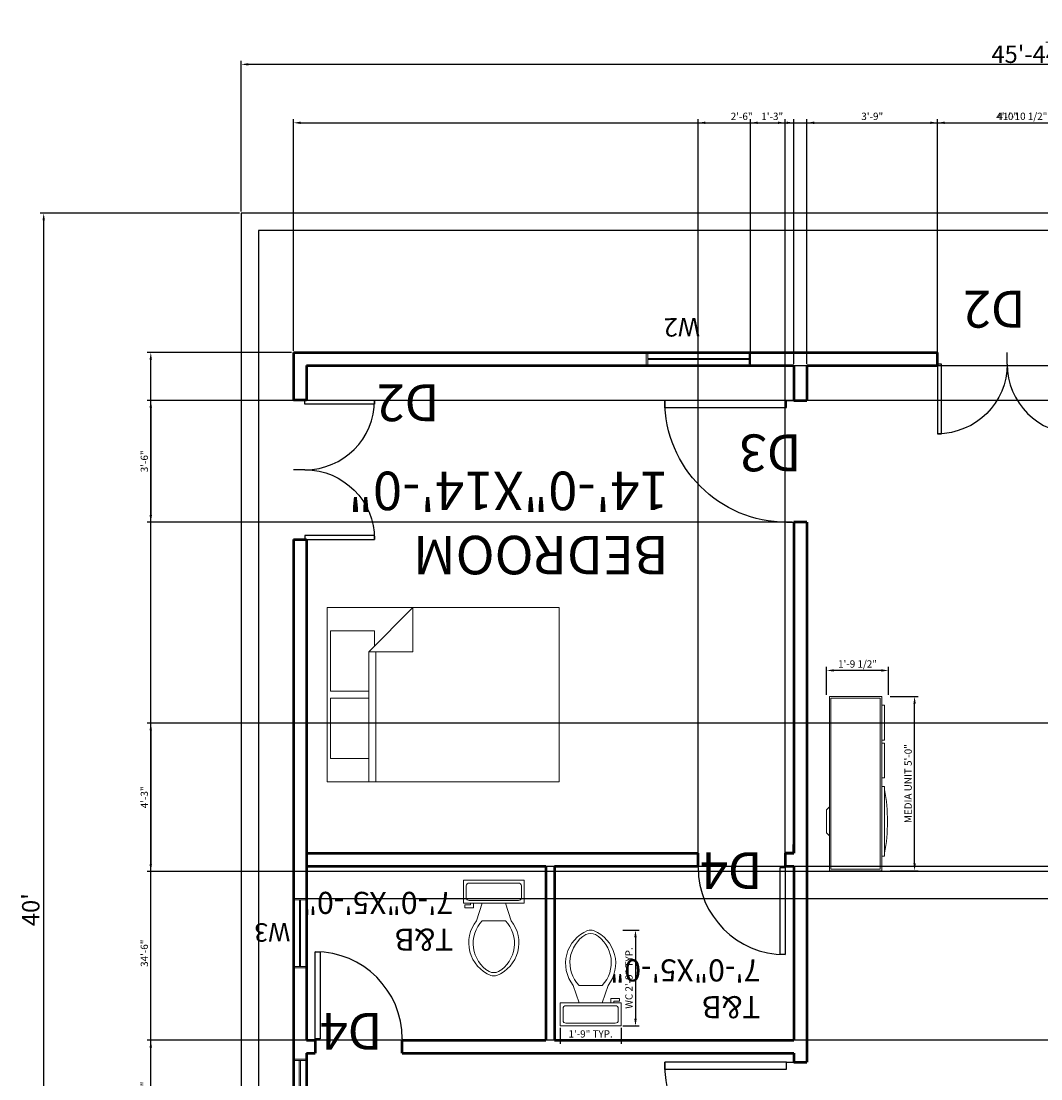
# Model space of a CAD drawing. Units: inches. Extents: x 1989 to 2637, y 1032 to 1611.
# Tile 2 of 5: x 1989 to 2340, y 1247 to 1611. Entities that reach past the tile are written whole.
import ezdxf

# ---------------------------------------------------------------- set-up
doc = ezdxf.new("R2010")
doc.units = ezdxf.units.IN
for name, color, linetype, lineweight in [('A-ANNO-TEXT', 1, 'Continuous', 18), ('A-AREA-IDEN', 1, 'Continuous', 25), ('A-FLOR-FIXT', 8, 'Continuous', 18), ('C-PROP', 7, 'Continuous', 25), ('DIMENSIONS', 7, 'Continuous', 18), ('doors', 5, 'Continuous', 25), ('furniture', 8, 'Continuous', 18), ('walls', 7, 'Continuous', 50), ('windows', 3, 'Continuous', 18)]:
    doc.layers.add(name, color=color, linetype=linetype, lineweight=lineweight)
doc.styles.get("Standard").update_dxf_attribs({"font": 'arial.ttf'})
doc.dimstyles.new('ISO-25', dxfattribs={"dimtxt": 2.5, "dimasz": 2.5, "dimexe": 1.25, "dimexo": 0.625, "dimtad": 1, "dimlunit": 4, "dimtxsty": 'Standard', "dimcen": 2.5, "dimadec": 0, "dimazin": 0, "dimtfac": 1, "dimtmove": 0, "dimatfit": 3, "dimfxl": 1, "dimarcsym": 0})

# ---------------------------------------------------------------- blocks, each defined once
blk = doc.blocks.new('*U2')
for p, q in [((0, 0), (0, -5)), ((30, 0), (30, -5))]:
    blk.add_line(p, q)
blk.add_lwpolyline([(0, 0), (0, 30), (1.75, 30), (1.75, 0)], close=True)
blk.add_arc((0, 0), 30, 0, 90)
blk = doc.blocks.new('Entertainment Center')
for p, q in [((-4, 0), (-5, -1)), ((4, 0), (-4, 0)), ((5, -1), (4, 0)), ((-17, -19), (-17, -1)), ((-17, -1), (43, -1)), ((-16.5, -18.5), (-16.5, -1.5)), ((-16.5, -1.5), (42.5, -1.5)), ((42.5, -1.5), (42.5, -18.5)), ((43, -1), (43, -19)), ((43, -19), (-17, -19)), ((42.5, -18.5), (-16.5, -18.5)), ((-12, -20), (-12, -19)), ((12, -20), (-12, -20)), ((12, -19), (12, -20)), ((15, -20), (15, -19)), ((27, -20), (15, -20)), ((27, -19), (27, -20)), ((28, -20), (28, -19)), ((40, -20), (28, -20)), ((40, -19), (40, -20))]:
    blk.add_line(p, q)
blk.add_arc((0, 40), 61, 259.6111, 280.3889)
blk = doc.blocks.new('Bed - Queen')
for p, q in [((0, -80.00003), (0, 0)), ((0, 0), (59.99999, 0)), ((59.99999, 0), (59.99999, -80.00003)), ((7.99999, -1.2), (28.79998, -1.2)), ((7.99999, -14.4), (7.99999, -1.2)), ((28.79998, -1.2), (28.79998, -14.4)), ((31.19999, -1.2), (51.99999, -1.2)), ((31.19999, -14.4), (31.19999, -1.2)), ((51.99999, -1.2), (51.99999, -16.4)), ((0, -14.4), (44.8, -14.4)), ((59.99999, -29.6), (44.8, -14.4)), ((44.8, -14.4), (44.8, -29.6)), ((44.8, -16.8), (0, -16.8)), ((51.99999, -16.4), (46.79936, -16.4)), ((44.8, -29.6), (59.99999, -29.6)), ((59.99999, -80.00003), (0, -80.00003))]:
    blk.add_line(p, q)
blk = doc.blocks.new('Toilet - top')
for p, q in [((9.5, -6), (9.5, -2)), ((-10, -8.5), (-8, -8.5)), ((-10, -9.5), (-10, -8.5)), ((-7, -9.5), (-10, -9.5)), ((-8, -8.5), (-8, -8)), ((-7, -8), (-7, -9.5)), ((-4, -8), (-6, -14)), ((4, -8), (6, -14)), ((4, -14), (-4, -14))]:
    blk.add_line(p, q)
blk.add_lwpolyline([(10.5, -8), (10.5, 0), (-10.5, 0), (-10.5, -8)], close=True)
for points in [[(-9.5, -2), (-9.5, -6)], [(8.5, -1), (-8.5, -1)], [(-8.5, -7), (8.5, -7)]]:
    blk.add_lwpolyline(points)
for centre, radius, start, end in [((-8.62, -1.88), 0.884, 81.8699, 188.1301), ((8.62, -1.88), 0.884, 351.8699, 98.1301), ((-8.62, -6.12), 0.884, 171.8699, 278.1301), ((8.62, -6.12), 0.884, 261.8699, 8.1301), ((3.52, -21.58), 12.17, 141.4691, 247.9714), ((4.2, -21.82), 11.33, 136.3677, 238.9468), ((-3.52, -21.58), 12.17, 292.0284, 38.5307), ((-4.2, -21.82), 11.33, 301.053, 43.6321), ((0, -27.88), 4, 245.7318, 294.2682), ((0, -29), 4, 254.8605, 285.1395)]:
    blk.add_arc(centre, radius, start, end)
blk = doc.blocks.new('*D11')
at = {"layer": 'Defpoints', "color": 0, "transparency": 16777216}
for p in [(1996.45, 1544.92), (2064.5, 1544.92), (2064.5, 1064.92)]:
    blk.add_point(p, dxfattribs=at)
at = {"layer": 'DIMENSIONS', "color": 0, "lineweight": -2, "transparency": 16777216}
for p, q in [((2063.87, 1544.92), (1995.2, 1544.92)), ((1996.45, 1067.42), (1996.45, 1542.42)), ((2063.87, 1064.92), (1995.2, 1064.92))]:
    blk.add_line(p, q, dxfattribs=at)
at = {"layer": 'DIMENSIONS', "color": 0, "transparency": 16777216}
for points in [[(1996.03, 1542.42), (1996.87, 1542.42), (1996.45, 1544.92)], [(1996.03, 1067.42), (1996.87, 1067.42), (1996.45, 1064.92)]]:
    blk.add_solid(points, dxfattribs=at)
at = {"layer": 'DIMENSIONS', "color": 0, "transparency": 16777216, "insert": (1992.76, 1304.92), "char_height": 6, "attachment_point": 5, "rotation": 90}
blk.add_mtext("40'", dxfattribs=at)
blk = doc.blocks.new('*D12')
at = {"layer": 'Defpoints', "color": 0, "transparency": 16777216}
for p in [(2064.5, 1596.21), (2064.5, 1544.92), (2608.81, 1544.92)]:
    blk.add_point(p, dxfattribs=at)
at = {"layer": 'DIMENSIONS', "color": 0, "lineweight": -2, "transparency": 16777216}
for p, q in [((2064.5, 1545.55), (2064.5, 1597.46)), ((2608.81, 1545.55), (2608.81, 1597.46)), ((2606.31, 1596.21), (2067, 1596.21))]:
    blk.add_line(p, q, dxfattribs=at)
at = {"layer": 'DIMENSIONS', "color": 0, "transparency": 16777216}
for points in [[(2067, 1596.63), (2067, 1595.79), (2064.5, 1596.21)], [(2606.31, 1596.63), (2606.31, 1595.79), (2608.81, 1596.21)]]:
    blk.add_solid(points, dxfattribs=at)
at = {"layer": 'DIMENSIONS', "color": 0, "transparency": 16777216, "insert": (2336.65, 1603.9), "char_height": 6, "attachment_point": 5}
blk.add_mtext('45\'-4{\\H1x;\\S1/4;}"', dxfattribs=at)
blk = doc.blocks.new('WIN-W3-24IN')
for p, q in [((0, 0), (0, 23.95)), ((0, 23.95), (4.5, 23.95)), ((0, 23.45), (4.5, 23.45)), ((2.05, 23.45), (2.05, 0.5)), ((2.45, 23.45), (2.45, 0.5)), ((4.5, 23.95), (4.5, 0)), ((4.5, 0.5), (0, 0.5)), ((4.5, 0), (0, 0))]:
    blk.add_line(p, q)
blk = doc.blocks.new('WIN-W2-36IN')
for p, q in [((0, 0), (0, 35.95)), ((0, 35.95), (4.5, 35.95)), ((0, 35.45), (4.5, 35.45)), ((2.05, 35.45), (2.05, 0.5)), ((2.45, 35.45), (2.45, 0.5)), ((4.5, 35.95), (4.5, 0)), ((4.5, 0.5), (0, 0.5)), ((4.5, 0), (0, 0))]:
    blk.add_line(p, q)
blk = doc.blocks.new('*D32')
at = {"layer": 'Defpoints', "color": 0, "transparency": 16777216}
for p in [(2195.44, 1297.89), (2195.44, 1264.85), (2200.4, 1264.85)]:
    blk.add_point(p, dxfattribs=at)
at = {"layer": 'DIMENSIONS', "color": 0, "lineweight": -2, "transparency": 16777216}
for p, q in [((2196.07, 1297.89), (2201.65, 1297.89)), ((2200.4, 1295.39), (2200.4, 1267.35)), ((2196.07, 1264.85), (2201.65, 1264.85))]:
    blk.add_line(p, q, dxfattribs=at)
at = {"layer": 'DIMENSIONS', "color": 0, "transparency": 16777216}
for points in [[(2199.98, 1295.39), (2200.82, 1295.39), (2200.4, 1297.89)], [(2199.98, 1267.35), (2200.82, 1267.35), (2200.4, 1264.85)]]:
    blk.add_solid(points, dxfattribs=at)
at = {"layer": 'DIMENSIONS', "color": 0, "transparency": 16777216, "insert": (2198.48, 1281.37), "char_height": 2.5, "attachment_point": 5, "rotation": 90}
blk.add_mtext('WC 2\'-9" TYP.', dxfattribs=at)
blk = doc.blocks.new('*D33')
at = {"layer": 'Defpoints', "color": 0, "transparency": 16777216}
for p in [(2174.44, 1264.85), (2195.44, 1264.85), (2174.44, 1259.89)]:
    blk.add_point(p, dxfattribs=at)
at = {"layer": 'DIMENSIONS', "color": 0, "lineweight": -2, "transparency": 16777216}
for p, q in [((2174.44, 1264.22), (2174.44, 1258.64)), ((2195.44, 1264.22), (2195.44, 1258.64)), ((2192.94, 1259.89), (2176.94, 1259.89))]:
    blk.add_line(p, q, dxfattribs=at)
at = {"layer": 'DIMENSIONS', "color": 0, "transparency": 16777216}
for points in [[(2176.94, 1260.31), (2176.94, 1259.47), (2174.44, 1259.89)], [(2192.94, 1260.31), (2192.94, 1259.47), (2195.44, 1259.89)]]:
    blk.add_solid(points, dxfattribs=at)
at = {"layer": 'DIMENSIONS', "color": 0, "transparency": 16777216, "insert": (2184.94, 1261.79), "char_height": 2.5, "attachment_point": 5}
blk.add_mtext('1\'-9" TYP.', dxfattribs=at)
blk = doc.blocks.new('*D38')
at = {"layer": 'Defpoints', "color": 0, "transparency": 16777216}
for p in [(2287.6, 1378.36), (2296.6, 1378.36), (2287.6, 1318.36)]:
    blk.add_point(p, dxfattribs=at)
at = {"layer": 'DIMENSIONS', "color": 0, "lineweight": -2, "transparency": 16777216}
for p, q in [((2288.22, 1378.36), (2297.85, 1378.36)), ((2296.6, 1320.86), (2296.6, 1375.86)), ((2288.22, 1318.36), (2297.85, 1318.36))]:
    blk.add_line(p, q, dxfattribs=at)
at = {"layer": 'DIMENSIONS', "color": 0, "transparency": 16777216}
for points in [[(2296.18, 1375.86), (2297.01, 1375.86), (2296.6, 1378.36)], [(2296.18, 1320.86), (2297.01, 1320.86), (2296.6, 1318.36)]]:
    blk.add_solid(points, dxfattribs=at)
at = {"layer": 'DIMENSIONS', "color": 0, "transparency": 16777216, "insert": (2294.69, 1348.36), "char_height": 2.5, "attachment_point": 5, "rotation": 90}
blk.add_mtext('MEDIA UNIT 5\'-0"', dxfattribs=at)
blk = doc.blocks.new('*D39')
at = {"layer": 'Defpoints', "color": 0, "transparency": 16777216}
for p in [(2266.26, 1387.36), (2266.26, 1378.36), (2287.6, 1378.36)]:
    blk.add_point(p, dxfattribs=at)
at = {"layer": 'DIMENSIONS', "color": 0, "lineweight": -2, "transparency": 16777216}
for p, q in [((2266.26, 1378.98), (2266.26, 1388.61)), ((2285.1, 1387.36), (2268.76, 1387.36)), ((2287.6, 1378.98), (2287.6, 1388.61))]:
    blk.add_line(p, q, dxfattribs=at)
at = {"layer": 'DIMENSIONS', "color": 0, "transparency": 16777216}
for points in [[(2268.76, 1387.77), (2268.76, 1386.94), (2266.26, 1387.36)], [(2285.1, 1387.77), (2285.1, 1386.94), (2287.6, 1387.36)]]:
    blk.add_solid(points, dxfattribs=at)
at = {"layer": 'DIMENSIONS', "color": 0, "transparency": 16777216, "insert": (2276.93, 1389.27), "char_height": 2.5, "attachment_point": 5}
blk.add_mtext('1\'-9 1/2"', dxfattribs=at)
blk = doc.blocks.new('*D40')
at = {"layer": 'Defpoints', "color": 0, "transparency": 16777216}
for p in [(2585, 1576.07), (2082.5, 1496.92), (2585, 1310.92)]:
    blk.add_point(p, dxfattribs=at)
at = {"layer": 'DIMENSIONS', "color": 0, "lineweight": -2, "transparency": 16777216}
for p, q in [((2082.5, 1497.55), (2082.5, 1577.32)), ((2085, 1576.07), (2582.5, 1576.07)), ((2585, 1311.55), (2585, 1577.32))]:
    blk.add_line(p, q, dxfattribs=at)
at = {"layer": 'DIMENSIONS', "color": 0, "transparency": 16777216}
for points in [[(2085, 1576.49), (2085, 1575.65), (2082.5, 1576.07)], [(2582.5, 1576.49), (2582.5, 1575.65), (2585, 1576.07)]]:
    blk.add_solid(points, dxfattribs=at)
at = {"layer": 'DIMENSIONS', "color": 0, "transparency": 16777216, "insert": (2333.75, 1577.99), "char_height": 2.5, "attachment_point": 5}
blk.add_mtext('41\'-10 1/2"', dxfattribs=at)
blk = doc.blocks.new('*D41')
at = {"layer": 'Defpoints', "color": 0, "transparency": 16777216}
for p in [(2033.35, 1496.92), (2082.5, 1496.92), (2082.5, 1082.92)]:
    blk.add_point(p, dxfattribs=at)
at = {"layer": 'DIMENSIONS', "color": 0, "lineweight": -2, "transparency": 16777216}
for p, q in [((2081.87, 1496.92), (2032.1, 1496.92)), ((2033.35, 1085.42), (2033.35, 1494.42)), ((2081.87, 1082.92), (2032.1, 1082.92))]:
    blk.add_line(p, q, dxfattribs=at)
at = {"layer": 'DIMENSIONS', "color": 0, "transparency": 16777216}
for points in [[(2032.93, 1494.42), (2033.76, 1494.42), (2033.35, 1496.92)], [(2032.93, 1085.42), (2033.76, 1085.42), (2033.35, 1082.92)]]:
    blk.add_solid(points, dxfattribs=at)
at = {"layer": 'DIMENSIONS', "color": 0, "transparency": 16777216, "insert": (2031.45, 1289.92), "char_height": 2.5, "attachment_point": 5, "rotation": 90}
blk.add_mtext('34\'-6"', dxfattribs=at)
blk = doc.blocks.new('*D43')
at = {"layer": 'Defpoints', "color": 0, "transparency": 16777216}
for p in [(2255, 1480.42), (2033.35, 1438.42), (2255, 1438.42)]:
    blk.add_point(p, dxfattribs=at)
at = {"layer": 'DIMENSIONS', "color": 0, "lineweight": -2, "transparency": 16777216}
for p, q in [((2254.37, 1480.42), (2032.1, 1480.42)), ((2033.35, 1477.92), (2033.35, 1440.92)), ((2254.37, 1438.42), (2032.1, 1438.42))]:
    blk.add_line(p, q, dxfattribs=at)
at = {"layer": 'DIMENSIONS', "color": 0, "transparency": 16777216}
for points in [[(2032.93, 1477.92), (2033.76, 1477.92), (2033.35, 1480.42)], [(2032.93, 1440.92), (2033.76, 1440.92), (2033.35, 1438.42)]]:
    blk.add_solid(points, dxfattribs=at)
at = {"layer": 'DIMENSIONS', "color": 0, "transparency": 16777216, "insert": (2031.45, 1459.42), "char_height": 2.5, "attachment_point": 5, "rotation": 90}
blk.add_mtext('3\'-6"', dxfattribs=at)
blk = doc.blocks.new('*D44')
at = {"layer": 'Defpoints', "color": 0, "transparency": 16777216}
for p in [(2352.5, 1576.07), (2304.5, 1496.92), (2352.5, 1496.92)]:
    blk.add_point(p, dxfattribs=at)
at = {"layer": 'DIMENSIONS', "color": 0, "lineweight": -2, "transparency": 16777216}
for p, q in [((2304.5, 1497.55), (2304.5, 1577.32)), ((2307, 1576.07), (2350, 1576.07)), ((2352.5, 1497.55), (2352.5, 1577.32))]:
    blk.add_line(p, q, dxfattribs=at)
at = {"layer": 'DIMENSIONS', "color": 0, "transparency": 16777216}
for points in [[(2307, 1576.49), (2307, 1575.65), (2304.5, 1576.07)], [(2350, 1576.49), (2350, 1575.65), (2352.5, 1576.07)]]:
    blk.add_solid(points, dxfattribs=at)
at = {"layer": 'DIMENSIONS', "color": 0, "transparency": 16777216, "insert": (2328.5, 1577.97), "char_height": 2.5, "attachment_point": 5}
blk.add_mtext('4\'-0"', dxfattribs=at)
blk = doc.blocks.new('*D45')
at = {"layer": 'Defpoints', "color": 0, "transparency": 16777216}
for p in [(2252, 1576.07), (2222, 1319.92), (2252, 1319.92)]:
    blk.add_point(p, dxfattribs=at)
at = {"layer": 'DIMENSIONS', "color": 0, "lineweight": -2, "transparency": 16777216}
for p, q in [((2222, 1320.55), (2222, 1577.32)), ((2224.5, 1576.07), (2249.5, 1576.07)), ((2252, 1320.55), (2252, 1577.32))]:
    blk.add_line(p, q, dxfattribs=at)
at = {"layer": 'DIMENSIONS', "color": 0, "transparency": 16777216}
for points in [[(2224.5, 1576.49), (2224.5, 1575.65), (2222, 1576.07)], [(2249.5, 1576.49), (2249.5, 1575.65), (2252, 1576.07)]]:
    blk.add_solid(points, dxfattribs=at)
at = {"layer": 'DIMENSIONS', "color": 0, "transparency": 16777216, "insert": (2237, 1577.97), "char_height": 2.5, "attachment_point": 5}
blk.add_mtext('2\'-6"', dxfattribs=at)
blk = doc.blocks.new('*D49')
at = {"layer": 'Defpoints', "color": 0, "transparency": 16777216}
for p in [(2304.5, 1576.07), (2259.5, 1492.42), (2304.5, 1492.42)]:
    blk.add_point(p, dxfattribs=at)
at = {"layer": 'DIMENSIONS', "color": 0, "lineweight": -2, "transparency": 16777216}
for p, q in [((2259.5, 1493.05), (2259.5, 1577.32)), ((2262, 1576.07), (2302, 1576.07)), ((2304.5, 1493.05), (2304.5, 1577.32))]:
    blk.add_line(p, q, dxfattribs=at)
at = {"layer": 'DIMENSIONS', "color": 0, "transparency": 16777216}
for points in [[(2262, 1576.49), (2262, 1575.65), (2259.5, 1576.07)], [(2302, 1576.49), (2302, 1575.65), (2304.5, 1576.07)]]:
    blk.add_solid(points, dxfattribs=at)
at = {"layer": 'DIMENSIONS', "color": 0, "transparency": 16777216, "insert": (2282, 1577.97), "char_height": 2.5, "attachment_point": 5}
blk.add_mtext('3\'-9"', dxfattribs=at)
blk = doc.blocks.new('*D50')
at = {"layer": 'Defpoints', "color": 0, "transparency": 16777216}
for p in [(2087, 1492.42), (2087, 1480.5), (2635.65, 1480.5)]:
    blk.add_point(p, dxfattribs=at)
at = {"layer": 'DIMENSIONS', "color": 0, "lineweight": -2, "transparency": 16777216}
for p, q in [((2087.62, 1492.42), (2636.9, 1492.42)), ((2635.65, 1489.92), (2635.65, 1483)), ((2087.62, 1480.5), (2636.9, 1480.5))]:
    blk.add_line(p, q, dxfattribs=at)
at = {"layer": 'DIMENSIONS', "color": 0, "transparency": 16777216}
for points in [[(2635.23, 1489.92), (2636.06, 1489.92), (2635.65, 1492.42)], [(2635.23, 1483), (2636.06, 1483), (2635.65, 1480.5)]]:
    blk.add_solid(points, dxfattribs=at)
at = {"layer": 'DIMENSIONS', "color": 0, "transparency": 16777216, "insert": (2633.75, 1486.46), "char_height": 2.5, "attachment_point": 5, "rotation": 90}
blk.add_mtext('1\'-0"', dxfattribs=at)
blk = doc.blocks.new('*D55')
at = {"layer": 'Defpoints', "color": 0, "transparency": 16777216}
for p in [(2414.53, 1369.21), (2033.35, 1318.07), (2414.53, 1318.07)]:
    blk.add_point(p, dxfattribs=at)
at = {"layer": 'DIMENSIONS', "color": 0, "lineweight": -2, "transparency": 16777216}
for p, q in [((2413.9, 1369.21), (2032.1, 1369.21)), ((2033.35, 1366.71), (2033.35, 1320.57)), ((2413.9, 1318.07), (2032.1, 1318.07))]:
    blk.add_line(p, q, dxfattribs=at)
at = {"layer": 'DIMENSIONS', "color": 0, "transparency": 16777216}
for points in [[(2032.93, 1366.71), (2033.76, 1366.71), (2033.35, 1369.21)], [(2032.93, 1320.57), (2033.76, 1320.57), (2033.35, 1318.07)]]:
    blk.add_solid(points, dxfattribs=at)
at = {"layer": 'DIMENSIONS', "color": 0, "transparency": 16777216, "insert": (2031.45, 1343.64), "char_height": 2.5, "attachment_point": 5, "rotation": 90}
blk.add_mtext('4\'-3"', dxfattribs=at)
blk = doc.blocks.new('*D57')
at = {"layer": 'Defpoints', "color": 0, "transparency": 16777216}
for p in [(2255, 1576.07), (2240.06, 1492.42), (2255, 1492.42)]:
    blk.add_point(p, dxfattribs=at)
at = {"layer": 'DIMENSIONS', "color": 0, "lineweight": -2, "transparency": 16777216}
for p, q in [((2240.06, 1493.05), (2240.06, 1577.32)), ((2242.56, 1576.07), (2252.5, 1576.07)), ((2255, 1493.05), (2255, 1577.32))]:
    blk.add_line(p, q, dxfattribs=at)
at = {"layer": 'DIMENSIONS', "color": 0, "transparency": 16777216}
for points in [[(2242.56, 1576.49), (2242.56, 1575.65), (2240.06, 1576.07)], [(2252.5, 1576.49), (2252.5, 1575.65), (2255, 1576.07)]]:
    blk.add_solid(points, dxfattribs=at)
at = {"layer": 'DIMENSIONS', "color": 0, "transparency": 16777216, "insert": (2247.53, 1577.97), "char_height": 2.5, "attachment_point": 5}
blk.add_mtext('1\'-3"', dxfattribs=at)
blk = doc.blocks.new('*D59')
at = {"layer": 'Defpoints', "color": 0, "transparency": 16777216}
for p in [(2033.35, 1259.92), (2415.5, 1259.92), (2415.5, 1223.92)]:
    blk.add_point(p, dxfattribs=at)
at = {"layer": 'DIMENSIONS', "color": 0, "lineweight": -2, "transparency": 16777216}
for p, q in [((2414.87, 1259.92), (2032.1, 1259.92)), ((2033.35, 1226.42), (2033.35, 1257.42)), ((2414.87, 1223.92), (2032.1, 1223.92))]:
    blk.add_line(p, q, dxfattribs=at)
at = {"layer": 'DIMENSIONS', "color": 0, "transparency": 16777216}
for points in [[(2032.93, 1257.42), (2033.76, 1257.42), (2033.35, 1259.92)], [(2032.93, 1226.42), (2033.76, 1226.42), (2033.35, 1223.92)]]:
    blk.add_solid(points, dxfattribs=at)
at = {"layer": 'DIMENSIONS', "color": 0, "transparency": 16777216, "insert": (2031.45, 1241.92), "char_height": 2.5, "attachment_point": 5, "rotation": 90}
blk.add_mtext('3\'-0"', dxfattribs=at)
blk = doc.blocks.new('*D63')
at = {"layer": 'Defpoints', "color": 0, "transparency": 16777216}
for p in [(2087, 1319.92), (2635.65, 1319.92), (2087, 1308.78)]:
    blk.add_point(p, dxfattribs=at)
at = {"layer": 'DIMENSIONS', "color": 0, "lineweight": -2, "transparency": 16777216}
for p, q in [((2087.62, 1319.92), (2636.9, 1319.92)), ((2635.65, 1311.28), (2635.65, 1317.42)), ((2087.62, 1308.78), (2636.9, 1308.78))]:
    blk.add_line(p, q, dxfattribs=at)
at = {"layer": 'DIMENSIONS', "color": 0, "transparency": 16777216}
for points in [[(2635.23, 1317.42), (2636.06, 1317.42), (2635.65, 1319.92)], [(2635.23, 1311.28), (2636.06, 1311.28), (2635.65, 1308.78)]]:
    blk.add_solid(points, dxfattribs=at)
at = {"layer": 'DIMENSIONS', "color": 0, "transparency": 16777216, "insert": (2633.75, 1314.35), "char_height": 2.5, "attachment_point": 5, "rotation": 90}
blk.add_mtext('0\'-11"', dxfattribs=at)

msp = doc.modelspace()

# ---------------------------------------------------------------- linework, layer by layer
at = {"layer": 'C-PROP'}
for p, q in [((2604.498, 1544.921), (2064.498, 1544.921)), ((2064.498, 1544.921), (2064.498, 1064.921)), ((2070.498, 1538.921), (2070.498, 1070.921)), ((2598.498, 1538.921), (2070.498, 1538.921))]:
    msp.add_line(p, q, dxfattribs=at)
at = {"layer": 'walls'}
for p, q in [((2082.498, 1496.921), (2082.498, 1480.504)), ((2082.498, 1496.921), (2304.498, 1496.921)), ((2304.498, 1492.421), (2304.498, 1496.921)), ((2086.998, 1492.421), (2086.998, 1480.504)), ((2086.998, 1492.421), (2254.998, 1492.421)), ((2254.998, 1492.421), (2254.998, 1480.421)), ((2254.998, 1492.421), (2254.998, 1480.421)), ((2259.498, 1492.421), (2259.498, 1480.421)), ((2259.498, 1492.421), (2304.498, 1492.421)), ((2086.998, 1480.504), (2082.498, 1480.504)), ((2254.998, 1480.421), (2259.498, 1480.421)), ((2259.498, 1438.421), (2254.998, 1438.421)), ((2254.998, 1438.421), (2254.998, 1324.421)), ((2259.498, 1438.421), (2259.498, 1252.421)), ((2082.498, 1432.504), (2086.998, 1432.504)), ((2082.498, 1432.504), (2082.498, 1082.921)), ((2086.998, 1432.504), (2086.998, 1259.921)), ((2254.998, 1324.421), (2254.998, 1327.421)), ((2086.998, 1324.421), (2221.998, 1324.421)), ((2221.998, 1319.921), (2221.998, 1324.421)), ((2254.998, 1324.421), (2251.998, 1324.421)), ((2251.998, 1324.421), (2251.998, 1319.921)), ((2251.998, 1324.421), (2254.998, 1324.421)), ((2086.998, 1319.921), (2169.498, 1319.921)), ((2169.498, 1319.921), (2169.498, 1259.921)), ((2172.498, 1319.921), (2172.498, 1259.921)), ((2172.498, 1319.921), (2221.998, 1319.921)), ((2251.998, 1319.921), (2254.998, 1319.921)), ((2254.998, 1319.921), (2254.998, 1259.921)), ((2086.998, 1259.921), (2089.998, 1259.921)), ((2086.998, 1259.921), (2089.998, 1259.921)), ((2089.998, 1259.921), (2089.998, 1255.421)), ((2119.998, 1255.421), (2119.998, 1259.921)), ((2119.998, 1259.921), (2169.498, 1259.921)), ((2172.498, 1259.921), (2254.998, 1259.921)), ((2086.998, 1255.421), (2089.998, 1255.421)), ((2086.998, 1255.421), (2086.998, 1087.421)), ((2119.998, 1255.421), (2254.998, 1255.421)), ((2254.998, 1255.421), (2254.998, 1252.421)), ((2254.998, 1255.421), (2254.998, 1252.421)), ((2254.998, 1252.421), (2259.498, 1252.421))]:
    msp.add_line(p, q, dxfattribs=at)

# ---------------------------------------------------------------- block references
at = {"layer": 'A-FLOR-FIXT'}
msp.add_blockref('Toilet - top', (2151.579, 1315.111), dxfattribs=at)
at = {"layer": 'A-FLOR-FIXT', "rotation": 180.0000000000004}
msp.add_blockref('Toilet - top', (2184.943, 1264.846), dxfattribs=at)
at = {"layer": 'doors'}
for p, xscale, yscale, zscale, rotation in [((2304.498, 1492.921), -0.8, 0.8, 0.8, 180), ((2352.498, 1492.921), 0.8, 0.8, 0.8, 180), ((2086.498, 1480.504), 0.8, 0.8, 0.8, 270), ((2252.498, 1480.421), -1.399999999999999, 1.399999999999999, 1.399999999999999, 90), ((2086.498, 1432.504), -0.8, 0.8, 0.8, 270), ((2252.498, 1252.421), -1.399999999999999, 1.399999999999999, 1.399999999999999, 90)]:
    msp.add_blockref('*U2', p, dxfattribs=dict(at, xscale=xscale, yscale=yscale, zscale=zscale, rotation=rotation))
at = {"layer": 'doors', "rotation": 180}
msp.add_blockref('*U2', (2251.998, 1319.421), dxfattribs=at)
at = {"layer": 'doors'}
msp.add_blockref('*U2', (2089.998, 1260.421), dxfattribs=at)
at = {"layer": 'furniture', "rotation": 90}
for name, p in [('Bed - Queen', (2094.097, 1349.015)), ('Entertainment Center', (2266.262, 1335.356))]:
    msp.add_blockref(name, p, dxfattribs=at)
at = {"layer": 'windows', "rotation": 89.99999999999741}
msp.add_blockref('WIN-W2-36IN', (2240.062, 1492.421), dxfattribs=at)
at = {"layer": 'windows'}
for name, p in [('WIN-W3-24IN', (2082.498, 1284.828)), ('WIN-W2-36IN', (2082.48, 1217.461))]:
    msp.add_blockref(name, p, dxfattribs=at)

# ---------------------------------------------------------------- texts
at = {"layer": 'A-ANNO-TEXT', "attachment_point": 1}
for s, width, gutter_width, insert, char_height, rotation in [('D2', 3.801, 63.542, (2334.844, 1505.49), 12.7085, 180), ('W2', 5.29651, 31.753, (2222.637, 1502.519), 6.3507, 180.67334), ('D2', 3.801, 63.542, (2132.786, 1473.245), 12.7085, 180), ('D3', 3.801, 63.542, (2257.632, 1455.971), 12.7085, 180), ('D4', 3.801, 63.542, (2244.187, 1312.022), 12.7085, 180), ('W3', 5.29651, 31.753, (2081.441, 1294.01), 6.3507, 180.67334), ('D4', 3.801, 63.542, (2113.15, 1256.645), 12.7085, 180)]:
    msp.add_mtext_dynamic_manual_height_columns(s, width=width, gutter_width=gutter_width, heights=[0], dxfattribs=dict(at, insert=insert, char_height=char_height, rotation=rotation))
at = {"layer": 'A-AREA-IDEN', "insert": (2211.799, 1420.474), "char_height": 13.26964, "attachment_point": 1, "rotation": 180}
msp.add_mtext_dynamic_manual_height_columns('BEDROOM\\P14\'-0"X14\'-0"', width=13.72319, gutter_width=66.348, heights=[0], dxfattribs=at)
at = {"layer": 'A-AREA-IDEN', "char_height": 7.60673, "attachment_point": 1, "rotation": 180}
for insert in [(2137.544, 1290.784), (2243.448, 1267.515)]:
    msp.add_mtext('T&B\\P7\'-0"X5\'-0"', dxfattribs=dict(at, insert=insert))

# ---------------------------------------------------------------- dimensions: what is measured, and where the dimension line sits
at = {"layer": 'DIMENSIONS'}
for base, p1, p2, override, picture, middle in [((2064.498, 1596.209), (2608.808, 1544.921), (2064.498, 1544.921), {"dimtxt": 6, "dimclrd": 0, "dimclre": 0, "dimclrt": 0}, '*D12', (2336.653, 1603.898)), ((2584.998, 1576.071), (2082.498, 1496.921), (2584.998, 1310.921), {"dimdec": 1, "dimlfac": 1, "dimrnd": 0, "dimzin": 1, "dimdsep": 46, "dimlunit": 4, "dimfrac": 2}, '*D40', (2333.748, 1577.989)), ((2251.998, 1576.071), (2221.998, 1319.921), (2251.998, 1319.921), {"dimdec": 1, "dimlfac": 1, "dimrnd": 0, "dimzin": 1, "dimdsep": 46, "dimlunit": 4, "dimfrac": 2}, '*D45', (2236.998, 1577.972)), ((2254.998, 1576.071), (2240.062, 1492.421), (2254.998, 1492.421), {"dimdec": 1, "dimlfac": 1, "dimrnd": 0, "dimzin": 1, "dimdsep": 46, "dimlunit": 4, "dimfrac": 2}, '*D57', (2247.53, 1577.973)), ((2304.498, 1576.071), (2259.498, 1492.421), (2304.498, 1492.421), {"dimdec": 1, "dimlfac": 1, "dimrnd": 0, "dimzin": 1, "dimdsep": 46, "dimlunit": 4, "dimfrac": 2}, '*D49', (2281.998, 1577.973)), ((2352.498, 1576.071), (2304.498, 1496.921), (2352.498, 1496.921), {"dimdec": 1, "dimlfac": 1, "dimrnd": 0, "dimzin": 1, "dimdsep": 46, "dimlunit": 4, "dimfrac": 2}, '*D44', (2328.498, 1577.972))]:
    dim = msp.add_linear_dim(base=base, p1=p1, p2=p2, dimstyle='ISO-25', override=override, dxfattribs=at)
    dim.commit()
    dim.dimension.update_dxf_attribs({"geometry": picture, "text_midpoint": middle})
for base, p1, p2, angle, override, picture, middle in [((1996.449, 1544.921), (2064.498, 1064.921), (2064.498, 1544.921), 90, {"dimtxt": 6, "dimclrd": 0, "dimclre": 0, "dimclrt": 0}, '*D11', (1992.76, 1304.921)), ((2033.348, 1496.921), (2082.498, 1082.921), (2082.498, 1496.921), 90, {"dimdec": 1, "dimlfac": 1, "dimrnd": 0, "dimzin": 1, "dimdsep": 46, "dimlunit": 4, "dimfrac": 2}, '*D41', (2031.445, 1289.921)), ((2635.648, 1480.504), (2086.998, 1492.421), (2086.998, 1480.504), 90, {"dimdec": 1, "dimlfac": 1, "dimrnd": 0, "dimzin": 1, "dimdsep": 46, "dimlunit": 4, "dimfrac": 2}, '*D50', (2633.746, 1486.463)), ((2033.348, 1438.421), (2254.998, 1480.421), (2254.998, 1438.421), 90, {"dimdec": 1, "dimlfac": 1, "dimrnd": 0, "dimzin": 1, "dimdsep": 46, "dimlunit": 4, "dimfrac": 2}, '*D43', (2031.445, 1459.421)), ((2266.262, 1387.356), (2287.595, 1378.356), (2266.262, 1378.356), 180, {"dimdec": 1, "dimlfac": 1, "dimrnd": 0, "dimzin": 1, "dimdsep": 46, "dimlunit": 4, "dimfrac": 2}, '*D39', (2276.929, 1389.273)), ((2033.348, 1318.065), (2414.527, 1369.207), (2414.527, 1318.065), 90, {"dimdec": 1, "dimlfac": 1, "dimrnd": 0, "dimzin": 1, "dimdsep": 46, "dimlunit": 4, "dimfrac": 2}, '*D55', (2031.445, 1343.636)), ((2635.648, 1319.921), (2086.998, 1308.778), (2086.998, 1319.921), 90, {"dimdec": 1, "dimlfac": 1, "dimrnd": 0, "dimzin": 1, "dimdsep": 46, "dimlunit": 4, "dimfrac": 2}, '*D63', (2633.746, 1314.349)), ((2033.348, 1259.921), (2415.498, 1223.921), (2415.498, 1259.921), 90, {"dimdec": 1, "dimlfac": 1, "dimrnd": 0, "dimzin": 1, "dimdsep": 46, "dimlunit": 4, "dimfrac": 2}, '*D59', (2031.445, 1241.921))]:
    dim = msp.add_linear_dim(base=base, p1=p1, p2=p2, angle=angle, dimstyle='ISO-25', override=override, dxfattribs=at)
    dim.commit()
    dim.dimension.update_dxf_attribs({"geometry": picture, "text_midpoint": middle})
for base, p1, p2, angle, text, picture, middle in [((2296.595, 1378.356), (2287.595, 1318.356), (2287.595, 1378.356), 90, 'MEDIA UNIT <>', '*D38', (2294.694, 1348.356)), ((2200.4, 1264.846), (2195.443, 1297.892), (2195.443, 1264.846), 270, 'WC <> TYP.', '*D32', (2198.482, 1281.369)), ((2174.443, 1259.889), (2195.443, 1264.846), (2174.443, 1264.846), 180, '<> TYP.', '*D33', (2184.943, 1261.791))]:
    dim = msp.add_linear_dim(base=base, p1=p1, p2=p2, angle=angle, text=text, dimstyle='ISO-25', override={"dimdec": 1, "dimlfac": 1, "dimrnd": 0, "dimzin": 1, "dimdsep": 46, "dimlunit": 4, "dimfrac": 2}, dxfattribs=at)
    dim.commit()
    dim.dimension.update_dxf_attribs({"geometry": picture, "text_midpoint": middle})

doc.saveas('drawing.dxf')
